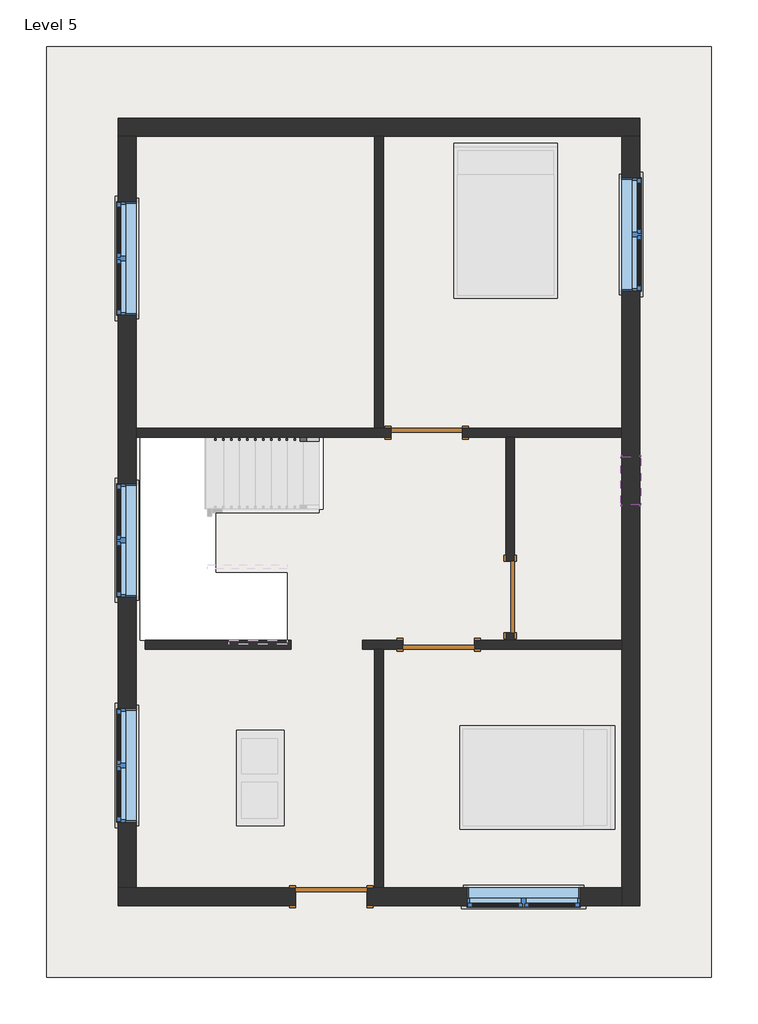
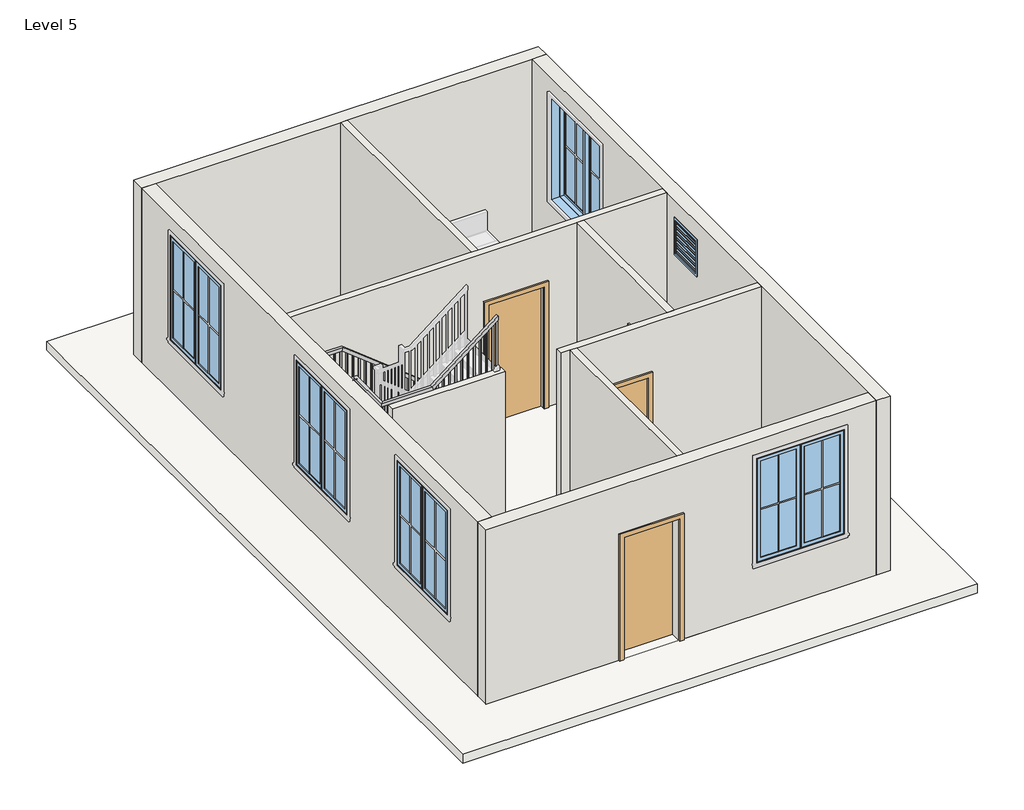
# One storey, part 1 of 2: 10 walls, 6 windows, 4 doors, 1 railing, 1 roof, 1 slab.
"""IFC4 building model written with IfcOpenShell, lengths in millimetres."""

from ifc_helpers import new_model, si_unit, frame, origin, place, context, project, spatial, polyline, outline, extrude, faceted_brep, transform, mapped, element, save
from components import door_e5f9f3c4, door_0ca8825f, window_9ac97e1a, window_f2d8fef0

model = new_model("IFC4")

# Units and contexts
model_context = context("Model", 3, world=origin())
ifc_project = project(units=[si_unit("LENGTHUNIT", "METRE", prefix="MILLI")], contexts=[model_context])

# Site, building, storey
site = spatial("IfcSite", under=ifc_project)
building = spatial("IfcBuilding", under=site)
storey = spatial("IfcBuildingStorey", under=building, Name="Level 5", Elevation=9601.2)

# Doors
placement = place(None, origin())
door_shape = door_e5f9f3c4(model_context)
element("IfcDoor", 1, ObjectType="Single-Flush : 36\" x 84\"", at=placement, inside=storey, context=model_context, shape_type="MappedRepresentation", body=[
    mapped(door_shape, transform((-2225.1840247, 979.1819954, 9601.2), x_axis=(1.0, 0.0, 0.0), y_axis=(0.0, 1.0, 0.0), z_axis=(0.0, 0.0, 1.0))),
])
element("IfcDoor", 2, ObjectType="Single-Flush : 36\" x 84\"", at=placement, inside=storey, context=model_context, shape_type="MappedRepresentation", body=[
    mapped(door_shape, transform((-1158.3840247, -1116.3180046, 9601.2), x_axis=(0.0, -1.0, 0.0), y_axis=(1.0, 0.0, 0.0), z_axis=(0.0, 0.0, 1.0))),
])
element("IfcDoor", 3, ObjectType="Single-Flush : 36\" x 84\"", at=placement, inside=storey, context=model_context, shape_type="MappedRepresentation", body=[
    mapped(door_shape, transform((-2072.7840247, -1725.9180046, 9601.2), x_axis=(-1.0, 0.0, 0.0), y_axis=(0.0, -1.0, 0.0), z_axis=(0.0, 0.0, 1.0))),
])
door_2_shape = door_0ca8825f(model_context)
element("IfcDoor", 4, ObjectType="Single-Flush : 36\" x 84\"", at=placement, inside=storey, context=model_context, shape_type="MappedRepresentation", body=[
    mapped(door_2_shape, transform((-3444.3840247, -4945.3680046, 9601.2), x_axis=(1.0, 0.0, 0.0), y_axis=(0.0, 1.0, 0.0), z_axis=(0.0, 0.0, 1.0))),
])

# Railing
element("IfcRailing", 5, ObjectType="Handrail - Rectangular", at=placement, inside=storey, context=model_context, shape_type="SolidModel", body=[
    faceted_brep([(-3603.1340247, 871.2319954, 10676.0210526), (-3603.1340247, 871.2319954, 10611.2980109), (-3603.1340247, 922.0319954, 10611.2980109), (-3603.1340247, 922.0319954, 10676.0210526), (-5097.5006913, 871.2319954, 11855.7842105), (-5115.1365442, 871.2319954, 11804.9842105), (-5115.1365442, 922.0319954, 11804.9842105), (-5097.5006913, 922.0319954, 11855.7842105), (-5889.1340247, 871.2319954, 11855.7842105), (-5889.1340247, 871.2319954, 11804.9842105), (-5939.9340247, 922.0319954, 11804.9842105), (-5939.9340247, 922.0319954, 11855.7842105), (-5889.1340247, 130.6632454, 11855.7842105), (-5889.1340247, 112.1228815, 11804.9842105), (-5939.9340247, 112.1228815, 11804.9842105), (-5939.9340247, 130.6632454, 11855.7842105), (-5889.1340247, -877.3992546, 12704.6789474), (-5889.1340247, -895.9396185, 12653.8789474), (-5939.9340247, -895.9396185, 12653.8789474), (-5939.9340247, -877.3992546, 12704.6789474), (-5889.1340247, -1617.9680046, 12704.6789474), (-5889.1340247, -1617.9680046, 12653.8789474), (-5939.9340247, -1668.7680046, 12653.8789474), (-5939.9340247, -1668.7680046, 12704.6789474), (-5097.5006913, -1617.9680046, 12704.6789474), (-5079.8648385, -1617.9680046, 12653.8789474), (-5079.8648385, -1668.7680046, 12653.8789474), (-5097.5006913, -1668.7680046, 12704.6789474), (-4009.5340247, -1617.9680046, 13563.6), (-4009.5340247, -1668.7680046, 13563.6), (-4009.5340247, -1668.7680046, 13498.8769583), (-4009.5340247, -1617.9680046, 13498.8769583)], [[[0, 1, 2, 3]], [[1, 0, 4, 5]], [[2, 1, 5, 6]], [[3, 2, 6, 7]], [[0, 3, 7, 4]], [[5, 4, 8, 9]], [[6, 5, 9, 10]], [[7, 6, 10, 11]], [[4, 7, 11, 8]], [[9, 8, 12, 13]], [[10, 9, 13, 14]], [[11, 10, 14, 15]], [[8, 11, 15, 12]], [[13, 12, 16, 17]], [[14, 13, 17, 18]], [[15, 14, 18, 19]], [[12, 15, 19, 16]], [[17, 16, 20, 21]], [[18, 17, 21, 22]], [[19, 18, 22, 23]], [[16, 19, 23, 20]], [[21, 20, 24, 25]], [[22, 21, 25, 26]], [[23, 22, 26, 27]], [[20, 23, 27, 24]], [[28, 29, 30, 31]], [[25, 24, 28, 31]], [[26, 25, 31, 30]], [[27, 26, 30, 29]], [[24, 27, 29, 28]]]),
    extrude(outline(polyline([(13446.2388004, -4076.2090247), (13431.1993267, -4095.2590247), (12488.7789474, -4095.2590247), (12488.7789474, -4076.2090247), (13446.2388004, -4076.2090247)])), frame((0.0, -1652.8930046, 0.0), z_axis=(0.0, 1.0, 0.0), x_axis=(0.0, 0.0, 1.0)), (0.0, 0.0, 1.0), 19.05),
    extrude(outline(polyline([(13366.028274, -4177.8090247), (13350.9888004, -4196.8590247), (12488.7789474, -4196.8590247), (12488.7789474, -4177.8090247), (13366.028274, -4177.8090247)])), frame((0.0, -1652.8930046, 0.0), z_axis=(0.0, 1.0, 0.0), x_axis=(0.0, 0.0, 1.0)), (0.0, 0.0, 1.0), 19.05),
    extrude(outline(polyline([(13285.8177477, -4279.4090247), (13270.778274, -4298.4590247), (12328.3578947, -4298.4590247), (12328.3578947, -4279.4090247), (13285.8177477, -4279.4090247)])), frame((0.0, -1652.8930046, 0.0), z_axis=(0.0, 1.0, 0.0), x_axis=(0.0, 0.0, 1.0)), (0.0, 0.0, 1.0), 19.05),
    extrude(outline(polyline([(13205.6072214, -4381.0090247), (13190.5677477, -4400.0590247), (12328.3578947, -4400.0590247), (12328.3578947, -4381.0090247), (13205.6072214, -4381.0090247)])), frame((0.0, -1652.8930046, 0.0), z_axis=(0.0, 1.0, 0.0), x_axis=(0.0, 0.0, 1.0)), (0.0, 0.0, 1.0), 19.05),
    extrude(outline(polyline([(13125.3966951, -4482.6090247), (13110.3572214, -4501.6590247), (12167.9368421, -4501.6590247), (12167.9368421, -4482.6090247), (13125.3966951, -4482.6090247)])), frame((0.0, -1652.8930046, 0.0), z_axis=(0.0, 1.0, 0.0), x_axis=(0.0, 0.0, 1.0)), (0.0, 0.0, 1.0), 19.05),
    extrude(outline(polyline([(13045.1861688, -4584.2090247), (13030.1466951, -4603.2590247), (12167.9368421, -4603.2590247), (12167.9368421, -4584.2090247), (13045.1861688, -4584.2090247)])), frame((0.0, -1652.8930046, 0.0), z_axis=(0.0, 1.0, 0.0), x_axis=(0.0, 0.0, 1.0)), (0.0, 0.0, 1.0), 19.05),
    extrude(outline(polyline([(12964.9756425, -4685.8090247), (12949.9361688, -4704.8590247), (12007.5157895, -4704.8590247), (12007.5157895, -4685.8090247), (12964.9756425, -4685.8090247)])), frame((0.0, -1652.8930046, 0.0), z_axis=(0.0, 1.0, 0.0), x_axis=(0.0, 0.0, 1.0)), (0.0, 0.0, 1.0), 19.05),
    extrude(outline(polyline([(12884.7651161, -4787.4090247), (12869.7256425, -4806.4590247), (12007.5157895, -4806.4590247), (12007.5157895, -4787.4090247), (12884.7651161, -4787.4090247)])), frame((0.0, -1652.8930046, 0.0), z_axis=(0.0, 1.0, 0.0), x_axis=(0.0, 0.0, 1.0)), (0.0, 0.0, 1.0), 19.05),
    extrude(outline(polyline([(12804.5545898, -4889.0090247), (12789.5151161, -4908.0590247), (11847.0947368, -4908.0590247), (11847.0947368, -4889.0090247), (12804.5545898, -4889.0090247)])), frame((0.0, -1652.8930046, 0.0), z_axis=(0.0, 1.0, 0.0), x_axis=(0.0, 0.0, 1.0)), (0.0, 0.0, 1.0), 19.05),
    extrude(outline(polyline([(12724.3440635, -4990.6090247), (12709.3045898, -5009.6590247), (11847.0947368, -5009.6590247), (11847.0947368, -4990.6090247), (12724.3440635, -4990.6090247)])), frame((0.0, -1652.8930046, 0.0), z_axis=(0.0, 1.0, 0.0), x_axis=(0.0, 0.0, 1.0)), (0.0, 0.0, 1.0), 19.05),
    extrude(outline(polyline([(-5111.2590247, -1652.8930046), (-5111.2590247, -1633.8430046), (-5092.2090247, -1633.8430046), (-5092.2090247, -1652.8930046), (-5111.2590247, -1652.8930046)])), frame((0.0, 0.0, 11686.6736842), z_axis=(0.0, 0.0, 1.0), x_axis=(1.0, 0.0, 0.0)), (0.0, 0.0, 1.0), 967.2052632),
    extrude(outline(polyline([(-5212.8590247, -1652.8930046), (-5212.8590247, -1633.8430046), (-5193.8090247, -1633.8430046), (-5193.8090247, -1652.8930046), (-5212.8590247, -1652.8930046)])), frame((0.0, 0.0, 11686.6736842), z_axis=(0.0, 0.0, 1.0), x_axis=(1.0, 0.0, 0.0)), (0.0, 0.0, 1.0), 967.2052632),
    extrude(outline(polyline([(-5314.4590247, -1652.8930046), (-5314.4590247, -1633.8430046), (-5295.4090247, -1633.8430046), (-5295.4090247, -1652.8930046), (-5314.4590247, -1652.8930046)])), frame((0.0, 0.0, 11686.6736842), z_axis=(0.0, 0.0, 1.0), x_axis=(1.0, 0.0, 0.0)), (0.0, 0.0, 1.0), 967.2052632),
    extrude(outline(polyline([(-5416.0590247, -1652.8930046), (-5416.0590247, -1633.8430046), (-5397.0090247, -1633.8430046), (-5397.0090247, -1652.8930046), (-5416.0590247, -1652.8930046)])), frame((0.0, 0.0, 11686.6736842), z_axis=(0.0, 0.0, 1.0), x_axis=(1.0, 0.0, 0.0)), (0.0, 0.0, 1.0), 967.2052632),
    extrude(outline(polyline([(-5517.6590247, -1652.8930046), (-5517.6590247, -1633.8430046), (-5498.6090247, -1633.8430046), (-5498.6090247, -1652.8930046), (-5517.6590247, -1652.8930046)])), frame((0.0, 0.0, 11686.6736842), z_axis=(0.0, 0.0, 1.0), x_axis=(1.0, 0.0, 0.0)), (0.0, 0.0, 1.0), 967.2052632),
    extrude(outline(polyline([(-5619.2590247, -1652.8930046), (-5619.2590247, -1633.8430046), (-5600.2090247, -1633.8430046), (-5600.2090247, -1652.8930046), (-5619.2590247, -1652.8930046)])), frame((0.0, 0.0, 11686.6736842), z_axis=(0.0, 0.0, 1.0), x_axis=(1.0, 0.0, 0.0)), (0.0, 0.0, 1.0), 967.2052632),
    extrude(outline(polyline([(-5720.8590247, -1652.8930046), (-5720.8590247, -1633.8430046), (-5701.8090247, -1633.8430046), (-5701.8090247, -1652.8930046), (-5720.8590247, -1652.8930046)])), frame((0.0, 0.0, 11686.6736842), z_axis=(0.0, 0.0, 1.0), x_axis=(1.0, 0.0, 0.0)), (0.0, 0.0, 1.0), 967.2052632),
    extrude(outline(polyline([(-5822.4590247, -1652.8930046), (-5822.4590247, -1633.8430046), (-5803.4090247, -1633.8430046), (-5803.4090247, -1652.8930046), (-5822.4590247, -1652.8930046)])), frame((0.0, 0.0, 11686.6736842), z_axis=(0.0, 0.0, 1.0), x_axis=(1.0, 0.0, 0.0)), (0.0, 0.0, 1.0), 967.2052632),
    extrude(outline(polyline([(-5924.0590247, -1532.2430046), (-5905.0090247, -1532.2430046), (-5905.0090247, -1551.2930046), (-5924.0590247, -1551.2930046), (-5924.0590247, -1532.2430046)])), frame((0.0, 0.0, 11686.6736842), z_axis=(0.0, 0.0, 1.0), x_axis=(1.0, 0.0, 0.0)), (0.0, 0.0, 1.0), 967.2052632),
    extrude(outline(polyline([(-5924.0590247, -1430.6430046), (-5905.0090247, -1430.6430046), (-5905.0090247, -1449.6930046), (-5924.0590247, -1449.6930046), (-5924.0590247, -1430.6430046)])), frame((0.0, 0.0, 11686.6736842), z_axis=(0.0, 0.0, 1.0), x_axis=(1.0, 0.0, 0.0)), (0.0, 0.0, 1.0), 967.2052632),
    extrude(outline(polyline([(-5924.0590247, -1329.0430046), (-5905.0090247, -1329.0430046), (-5905.0090247, -1348.0930046), (-5924.0590247, -1348.0930046), (-5924.0590247, -1329.0430046)])), frame((0.0, 0.0, 11686.6736842), z_axis=(0.0, 0.0, 1.0), x_axis=(1.0, 0.0, 0.0)), (0.0, 0.0, 1.0), 967.2052632),
    extrude(outline(polyline([(-5924.0590247, -1227.4430046), (-5905.0090247, -1227.4430046), (-5905.0090247, -1246.4930046), (-5924.0590247, -1246.4930046), (-5924.0590247, -1227.4430046)])), frame((0.0, 0.0, 11686.6736842), z_axis=(0.0, 0.0, 1.0), x_axis=(1.0, 0.0, 0.0)), (0.0, 0.0, 1.0), 967.2052632),
    extrude(outline(polyline([(-5924.0590247, -1125.8430046), (-5905.0090247, -1125.8430046), (-5905.0090247, -1144.8930046), (-5924.0590247, -1144.8930046), (-5924.0590247, -1125.8430046)])), frame((0.0, 0.0, 11686.6736842), z_axis=(0.0, 0.0, 1.0), x_axis=(1.0, 0.0, 0.0)), (0.0, 0.0, 1.0), 967.2052632),
    extrude(outline(polyline([(-5924.0590247, -1024.2430046), (-5905.0090247, -1024.2430046), (-5905.0090247, -1043.2930046), (-5924.0590247, -1043.2930046), (-5924.0590247, -1024.2430046)])), frame((0.0, 0.0, 11686.6736842), z_axis=(0.0, 0.0, 1.0), x_axis=(1.0, 0.0, 0.0)), (0.0, 0.0, 1.0), 967.2052632),
    extrude(outline(polyline([(-5924.0590247, -922.6430046), (-5905.0090247, -922.6430046), (-5905.0090247, -941.6930046), (-5924.0590247, -941.6930046), (-5924.0590247, -922.6430046)])), frame((0.0, 0.0, 11686.6736842), z_axis=(0.0, 0.0, 1.0), x_axis=(1.0, 0.0, 0.0)), (0.0, 0.0, 1.0), 967.2052632),
    extrude(outline(polyline([(-840.0930046, 12606.8502199), (-821.0430046, 12590.8081146), (-821.0430046, 11686.6736842), (-840.0930046, 11686.6736842), (-840.0930046, 12606.8502199)])), frame((-5924.0590247, 0.0, 0.0), z_axis=(1.0, 0.0, 0.0), x_axis=(0.0, 1.0, 0.0)), (0.0, 0.0, 1.0), 19.05),
    extrude(outline(polyline([(-738.4930046, 12521.2923251), (-719.4430046, 12505.2502199), (-719.4430046, 11526.2526316), (-738.4930046, 11526.2526316), (-738.4930046, 12521.2923251)])), frame((-5924.0590247, 0.0, 0.0), z_axis=(1.0, 0.0, 0.0), x_axis=(0.0, 1.0, 0.0)), (0.0, 0.0, 1.0), 19.05),
    extrude(outline(polyline([(-636.8930046, 12435.7344304), (-617.8430046, 12419.6923251), (-617.8430046, 11526.2526316), (-636.8930046, 11526.2526316), (-636.8930046, 12435.7344304)])), frame((-5924.0590247, 0.0, 0.0), z_axis=(1.0, 0.0, 0.0), x_axis=(0.0, 1.0, 0.0)), (0.0, 0.0, 1.0), 19.05),
    extrude(outline(polyline([(-535.2930046, 12350.1765357), (-516.2430046, 12334.1344304), (-516.2430046, 11365.8315789), (-535.2930046, 11365.8315789), (-535.2930046, 12350.1765357)])), frame((-5924.0590247, 0.0, 0.0), z_axis=(1.0, 0.0, 0.0), x_axis=(0.0, 1.0, 0.0)), (0.0, 0.0, 1.0), 19.05),
    extrude(outline(polyline([(-433.6930046, 12264.6186409), (-414.6430046, 12248.5765357), (-414.6430046, 11365.8315789), (-433.6930046, 11365.8315789), (-433.6930046, 12264.6186409)])), frame((-5924.0590247, 0.0, 0.0), z_axis=(1.0, 0.0, 0.0), x_axis=(0.0, 1.0, 0.0)), (0.0, 0.0, 1.0), 19.05),
    extrude(outline(polyline([(-332.0930046, 12179.0607462), (-313.0430046, 12163.0186409), (-313.0430046, 11205.4105263), (-332.0930046, 11205.4105263), (-332.0930046, 12179.0607462)])), frame((-5924.0590247, 0.0, 0.0), z_axis=(1.0, 0.0, 0.0), x_axis=(0.0, 1.0, 0.0)), (0.0, 0.0, 1.0), 19.05),
    extrude(outline(polyline([(-230.4930046, 12093.5028514), (-211.4430046, 12077.4607462), (-211.4430046, 11205.4105263), (-230.4930046, 11205.4105263), (-230.4930046, 12093.5028514)])), frame((-5924.0590247, 0.0, 0.0), z_axis=(1.0, 0.0, 0.0), x_axis=(0.0, 1.0, 0.0)), (0.0, 0.0, 1.0), 19.05),
    extrude(outline(polyline([(-128.8930046, 12007.9449567), (-109.8430046, 11991.9028514), (-109.8430046, 11044.9894737), (-128.8930046, 11044.9894737), (-128.8930046, 12007.9449567)])), frame((-5924.0590247, 0.0, 0.0), z_axis=(1.0, 0.0, 0.0), x_axis=(0.0, 1.0, 0.0)), (0.0, 0.0, 1.0), 19.05),
    extrude(outline(polyline([(-27.2930046, 11922.387062), (-8.2430046, 11906.3449567), (-8.2430046, 11044.9894737), (-27.2930046, 11044.9894737), (-27.2930046, 11922.387062)])), frame((-5924.0590247, 0.0, 0.0), z_axis=(1.0, 0.0, 0.0), x_axis=(0.0, 1.0, 0.0)), (0.0, 0.0, 1.0), 19.05),
    extrude(outline(polyline([(74.3069954, 11836.8291672), (93.3569954, 11820.787062), (93.3569954, 10884.5684211), (74.3069954, 10884.5684211), (74.3069954, 11836.8291672)])), frame((-5924.0590247, 0.0, 0.0), z_axis=(1.0, 0.0, 0.0), x_axis=(0.0, 1.0, 0.0)), (0.0, 0.0, 1.0), 19.05),
    extrude(outline(polyline([(-5924.0590247, 194.9569954), (-5905.0090247, 194.9569954), (-5905.0090247, 175.9069954), (-5924.0590247, 175.9069954), (-5924.0590247, 194.9569954)])), frame((0.0, 0.0, 10884.5684211), z_axis=(0.0, 0.0, 1.0), x_axis=(1.0, 0.0, 0.0)), (0.0, 0.0, 1.0), 920.4157895),
    extrude(outline(polyline([(-5924.0590247, 296.5569954), (-5905.0090247, 296.5569954), (-5905.0090247, 277.5069954), (-5924.0590247, 277.5069954), (-5924.0590247, 296.5569954)])), frame((0.0, 0.0, 10884.5684211), z_axis=(0.0, 0.0, 1.0), x_axis=(1.0, 0.0, 0.0)), (0.0, 0.0, 1.0), 920.4157895),
    extrude(outline(polyline([(-5924.0590247, 398.1569954), (-5905.0090247, 398.1569954), (-5905.0090247, 379.1069954), (-5924.0590247, 379.1069954), (-5924.0590247, 398.1569954)])), frame((0.0, 0.0, 10884.5684211), z_axis=(0.0, 0.0, 1.0), x_axis=(1.0, 0.0, 0.0)), (0.0, 0.0, 1.0), 920.4157895),
    extrude(outline(polyline([(-5924.0590247, 499.7569954), (-5905.0090247, 499.7569954), (-5905.0090247, 480.7069954), (-5924.0590247, 480.7069954), (-5924.0590247, 499.7569954)])), frame((0.0, 0.0, 10884.5684211), z_axis=(0.0, 0.0, 1.0), x_axis=(1.0, 0.0, 0.0)), (0.0, 0.0, 1.0), 920.4157895),
    extrude(outline(polyline([(-5924.0590247, 601.3569954), (-5905.0090247, 601.3569954), (-5905.0090247, 582.3069954), (-5924.0590247, 582.3069954), (-5924.0590247, 601.3569954)])), frame((0.0, 0.0, 10884.5684211), z_axis=(0.0, 0.0, 1.0), x_axis=(1.0, 0.0, 0.0)), (0.0, 0.0, 1.0), 920.4157895),
    extrude(outline(polyline([(-5924.0590247, 702.9569954), (-5905.0090247, 702.9569954), (-5905.0090247, 683.9069954), (-5924.0590247, 683.9069954), (-5924.0590247, 702.9569954)])), frame((0.0, 0.0, 10884.5684211), z_axis=(0.0, 0.0, 1.0), x_axis=(1.0, 0.0, 0.0)), (0.0, 0.0, 1.0), 920.4157895),
    extrude(outline(polyline([(-5924.0590247, 804.5569954), (-5905.0090247, 804.5569954), (-5905.0090247, 785.5069954), (-5924.0590247, 785.5069954), (-5924.0590247, 804.5569954)])), frame((0.0, 0.0, 10884.5684211), z_axis=(0.0, 0.0, 1.0), x_axis=(1.0, 0.0, 0.0)), (0.0, 0.0, 1.0), 920.4157895),
    extrude(outline(polyline([(-5828.8090247, 906.1569954), (-5828.8090247, 887.1069954), (-5847.8590247, 887.1069954), (-5847.8590247, 906.1569954), (-5828.8090247, 906.1569954)])), frame((0.0, 0.0, 10884.5684211), z_axis=(0.0, 0.0, 1.0), x_axis=(1.0, 0.0, 0.0)), (0.0, 0.0, 1.0), 920.4157895),
    extrude(outline(polyline([(-5727.2090247, 906.1569954), (-5727.2090247, 887.1069954), (-5746.2590247, 887.1069954), (-5746.2590247, 906.1569954), (-5727.2090247, 906.1569954)])), frame((0.0, 0.0, 10884.5684211), z_axis=(0.0, 0.0, 1.0), x_axis=(1.0, 0.0, 0.0)), (0.0, 0.0, 1.0), 920.4157895),
    extrude(outline(polyline([(-5625.6090247, 906.1569954), (-5625.6090247, 887.1069954), (-5644.6590247, 887.1069954), (-5644.6590247, 906.1569954), (-5625.6090247, 906.1569954)])), frame((0.0, 0.0, 10884.5684211), z_axis=(0.0, 0.0, 1.0), x_axis=(1.0, 0.0, 0.0)), (0.0, 0.0, 1.0), 920.4157895),
    extrude(outline(polyline([(-5524.0090247, 906.1569954), (-5524.0090247, 887.1069954), (-5543.0590247, 887.1069954), (-5543.0590247, 906.1569954), (-5524.0090247, 906.1569954)])), frame((0.0, 0.0, 10884.5684211), z_axis=(0.0, 0.0, 1.0), x_axis=(1.0, 0.0, 0.0)), (0.0, 0.0, 1.0), 920.4157895),
    extrude(outline(polyline([(-5422.4090247, 906.1569954), (-5422.4090247, 887.1069954), (-5441.4590247, 887.1069954), (-5441.4590247, 906.1569954), (-5422.4090247, 906.1569954)])), frame((0.0, 0.0, 10884.5684211), z_axis=(0.0, 0.0, 1.0), x_axis=(1.0, 0.0, 0.0)), (0.0, 0.0, 1.0), 920.4157895),
    extrude(outline(polyline([(-5320.8090247, 906.1569954), (-5320.8090247, 887.1069954), (-5339.8590247, 887.1069954), (-5339.8590247, 906.1569954), (-5320.8090247, 906.1569954)])), frame((0.0, 0.0, 10884.5684211), z_axis=(0.0, 0.0, 1.0), x_axis=(1.0, 0.0, 0.0)), (0.0, 0.0, 1.0), 920.4157895),
    extrude(outline(polyline([(-5219.2090247, 906.1569954), (-5219.2090247, 887.1069954), (-5238.2590247, 887.1069954), (-5238.2590247, 906.1569954), (-5219.2090247, 906.1569954)])), frame((0.0, 0.0, 10884.5684211), z_axis=(0.0, 0.0, 1.0), x_axis=(1.0, 0.0, 0.0)), (0.0, 0.0, 1.0), 920.4157895),
    extrude(outline(polyline([(-5117.6090247, 906.1569954), (-5117.6090247, 887.1069954), (-5136.6590247, 887.1069954), (-5136.6590247, 906.1569954), (-5117.6090247, 906.1569954)])), frame((0.0, 0.0, 10884.5684211), z_axis=(0.0, 0.0, 1.0), x_axis=(1.0, 0.0, 0.0)), (0.0, 0.0, 1.0), 920.4157895),
    extrude(outline(polyline([(11726.7256425, -5016.0090247), (11741.7651161, -5035.0590247), (10884.5684211, -5035.0590247), (10884.5684211, -5016.0090247), (11726.7256425, -5016.0090247)])), frame((0.0, 887.1069954, 0.0), z_axis=(0.0, 1.0, 0.0), x_axis=(0.0, 0.0, 1.0)), (0.0, 0.0, 1.0), 19.05),
    extrude(outline(polyline([(11646.5151161, -4914.4090247), (11661.5545898, -4933.4590247), (10724.1473684, -4933.4590247), (10724.1473684, -4914.4090247), (11646.5151161, -4914.4090247)])), frame((0.0, 887.1069954, 0.0), z_axis=(0.0, 1.0, 0.0), x_axis=(0.0, 0.0, 1.0)), (0.0, 0.0, 1.0), 19.05),
    extrude(outline(polyline([(11566.3045898, -4812.8090247), (11581.3440635, -4831.8590247), (10724.1473684, -4831.8590247), (10724.1473684, -4812.8090247), (11566.3045898, -4812.8090247)])), frame((0.0, 887.1069954, 0.0), z_axis=(0.0, 1.0, 0.0), x_axis=(0.0, 0.0, 1.0)), (0.0, 0.0, 1.0), 19.05),
    extrude(outline(polyline([(11486.0940635, -4711.2090247), (11501.1335372, -4730.2590247), (10563.7263158, -4730.2590247), (10563.7263158, -4711.2090247), (11486.0940635, -4711.2090247)])), frame((0.0, 887.1069954, 0.0), z_axis=(0.0, 1.0, 0.0), x_axis=(0.0, 0.0, 1.0)), (0.0, 0.0, 1.0), 19.05),
    extrude(outline(polyline([(11405.8835372, -4609.6090247), (11420.9230109, -4628.6590247), (10563.7263158, -4628.6590247), (10563.7263158, -4609.6090247), (11405.8835372, -4609.6090247)])), frame((0.0, 887.1069954, 0.0), z_axis=(0.0, 1.0, 0.0), x_axis=(0.0, 0.0, 1.0)), (0.0, 0.0, 1.0), 19.05),
    extrude(outline(polyline([(11325.6730109, -4508.0090247), (11340.7124846, -4527.0590247), (10403.3052632, -4527.0590247), (10403.3052632, -4508.0090247), (11325.6730109, -4508.0090247)])), frame((0.0, 887.1069954, 0.0), z_axis=(0.0, 1.0, 0.0), x_axis=(0.0, 0.0, 1.0)), (0.0, 0.0, 1.0), 19.05),
    extrude(outline(polyline([(11245.4624846, -4406.4090247), (11260.5019583, -4425.4590247), (10403.3052632, -4425.4590247), (10403.3052632, -4406.4090247), (11245.4624846, -4406.4090247)])), frame((0.0, 887.1069954, 0.0), z_axis=(0.0, 1.0, 0.0), x_axis=(0.0, 0.0, 1.0)), (0.0, 0.0, 1.0), 19.05),
    extrude(outline(polyline([(11165.2519583, -4304.8090247), (11180.2914319, -4323.8590247), (10242.8842105, -4323.8590247), (10242.8842105, -4304.8090247), (11165.2519583, -4304.8090247)])), frame((0.0, 887.1069954, 0.0), z_axis=(0.0, 1.0, 0.0), x_axis=(0.0, 0.0, 1.0)), (0.0, 0.0, 1.0), 19.05),
    extrude(outline(polyline([(11085.0414319, -4203.2090247), (11100.0809056, -4222.2590247), (10242.8842105, -4222.2590247), (10242.8842105, -4203.2090247), (11085.0414319, -4203.2090247)])), frame((0.0, 887.1069954, 0.0), z_axis=(0.0, 1.0, 0.0), x_axis=(0.0, 0.0, 1.0)), (0.0, 0.0, 1.0), 19.05),
    extrude(outline(polyline([(11004.8309056, -4101.6090247), (11019.8703793, -4120.6590247), (10082.4631579, -4120.6590247), (10082.4631579, -4101.6090247), (11004.8309056, -4101.6090247)])), frame((0.0, 887.1069954, 0.0), z_axis=(0.0, 1.0, 0.0), x_axis=(0.0, 0.0, 1.0)), (0.0, 0.0, 1.0), 19.05),
    extrude(outline(polyline([(10924.6203793, -4000.0090247), (10939.659853, -4019.0590247), (10082.4631579, -4019.0590247), (10082.4631579, -4000.0090247), (10924.6203793, -4000.0090247)])), frame((0.0, 887.1069954, 0.0), z_axis=(0.0, 1.0, 0.0), x_axis=(0.0, 0.0, 1.0)), (0.0, 0.0, 1.0), 19.05),
    extrude(outline(polyline([(10844.409853, -3898.4090247), (10859.4493267, -3917.4590247), (9922.0421053, -3917.4590247), (9922.0421053, -3898.4090247), (10844.409853, -3898.4090247)])), frame((0.0, 887.1069954, 0.0), z_axis=(0.0, 1.0, 0.0), x_axis=(0.0, 0.0, 1.0)), (0.0, 0.0, 1.0), 19.05),
    extrude(outline(polyline([(10764.1993267, -3796.8090247), (10779.2388004, -3815.8590247), (9922.0421053, -3815.8590247), (9922.0421053, -3796.8090247), (10764.1993267, -3796.8090247)])), frame((0.0, 887.1069954, 0.0), z_axis=(0.0, 1.0, 0.0), x_axis=(0.0, 0.0, 1.0)), (0.0, 0.0, 1.0), 19.05),
    extrude(outline(polyline([(10683.9888004, -3695.2090247), (10699.028274, -3714.2590247), (9761.6210526, -3714.2590247), (9761.6210526, -3695.2090247), (10683.9888004, -3695.2090247)])), frame((0.0, 887.1069954, 0.0), z_axis=(0.0, 1.0, 0.0), x_axis=(0.0, 0.0, 1.0)), (0.0, 0.0, 1.0), 19.05),
    extrude(outline(polyline([(-5924.0590247, -1633.8430046), (-5905.0090247, -1633.8430046), (-5905.0090247, -1652.8930046), (-5924.0590247, -1652.8930046), (-5924.0590247, -1633.8430046)])), frame((0.0, 0.0, 11686.6736842), z_axis=(0.0, 0.0, 1.0), x_axis=(1.0, 0.0, 0.0)), (0.0, 0.0, 1.0), 967.2052632),
    extrude(outline(polyline([(-5905.0090247, 906.1569954), (-5905.0090247, 887.1069954), (-5924.0590247, 887.1069954), (-5924.0590247, 906.1569954), (-5905.0090247, 906.1569954)])), frame((0.0, 0.0, 10884.5684211), z_axis=(0.0, 0.0, 1.0), x_axis=(1.0, 0.0, 0.0)), (0.0, 0.0, 1.0), 920.4157895),
    extrude(outline(polyline([(13498.8769583, -4009.5340247), (13483.8374846, -4028.5840247), (12488.7789474, -4028.5840247), (12488.7789474, -4009.5340247), (13498.8769583, -4009.5340247)])), frame((0.0, -1652.8930046, 0.0), z_axis=(0.0, 1.0, 0.0), x_axis=(0.0, 0.0, 1.0)), (0.0, 0.0, 1.0), 19.05),
    extrude(outline(polyline([(10611.2980109, -3603.1340247), (10626.3374846, -3622.1840247), (9761.6210526, -3622.1840247), (9761.6210526, -3603.1340247), (10611.2980109, -3603.1340247)])), frame((0.0, 887.1069954, 0.0), z_axis=(0.0, 1.0, 0.0), x_axis=(0.0, 0.0, 1.0)), (0.0, 0.0, 1.0), 19.05),
])

# Roof
element("IfcRoof", 6, ObjectType="ROOF 6\"", at=placement, inside=storey, context=model_context, shape_type="SweptSolid", body=[
    extrude(outline(polyline([(-7082.9340247, 5913.1319954), (1413.3659753, 5913.1319954), (1413.3659753, -5974.0680046), (-7082.9340247, -5974.0680046), (-7082.9340247, 5913.1319954)]), holes=[polyline([(-5889.1340247, 922.0319954), (-5889.1340247, -1668.7680046), (-4009.5340247, -1668.7680046), (-4009.5340247, -805.1680046), (-4923.9340247, -805.1680046), (-4923.9340247, 7.6319954), (-3552.3340247, 7.6319954), (-3552.3340247, 922.0319954), (-5889.1340247, 922.0319954)])]), frame((0.0, 0.0, 9448.8), z_axis=(0.0, 0.0, 1.0), x_axis=(1.0, 0.0, 0.0)), (0.0, 0.0, 1.0), 152.4),
])

# Slab
element("IfcSlab", 7, ObjectType="FLOOR 6\"", at=placement, inside=storey, context=model_context, shape_type="SweptSolid", body=[
    extrude(outline(polyline([(498.9659753, 4998.7319954), (498.9659753, -5059.6680046), (-6168.5340247, -5059.6680046), (-6168.5340247, 4998.7319954), (498.9659753, 4998.7319954)]), holes=[polyline([(-5889.1340247, 922.0319954), (-5889.1340247, -1668.7680046), (-4009.5340247, -1668.7680046), (-4009.5340247, -805.1680046), (-4923.9340247, -805.1680046), (-4923.9340247, 7.6319954), (-3552.3340247, 7.6319954), (-3552.3340247, 922.0319954), (-5889.1340247, 922.0319954)])]), frame((0.0, 0.0, 9448.8), z_axis=(0.0, 0.0, 1.0), x_axis=(1.0, 0.0, 0.0)), (0.0, 0.0, 1.0), 152.4),
])

# Walls
element("IfcWall", 8, ObjectType="WALL 4.5\"", at=placement, inside=storey, context=model_context, shape_type="SweptSolid", body=[
    extrude(outline(polyline([(-2891.9340247, 1036.3319954), (-2891.9340247, 4770.1319954), (-2777.6340247, 4770.1319954), (-2777.6340247, 1036.3319954), (-2891.9340247, 1036.3319954)])), frame((0.0, 0.0, 9601.2), z_axis=(0.0, 0.0, 1.0), x_axis=(1.0, 0.0, 0.0)), (0.0, 0.0, 1.0), 3048.0),
])
element("IfcWall", 9, ObjectType="WALL 4.5\"", at=placement, inside=storey, context=model_context, shape_type="Brep", body=[
    faceted_brep([(-1767.9840247, 922.0319954, 11734.8), (-1767.9840247, 922.0319954, 9601.2), (-1215.5340247, 922.0319954, 9601.2), (-1101.2340247, 922.0319954, 9601.2), (270.3659753, 922.0319954, 9601.2), (270.3659753, 922.0319954, 12649.2), (-1101.2340247, 922.0319954, 12649.2), (-1215.5340247, 922.0319954, 12649.2), (-3552.3340247, 922.0319954, 12649.2), (-5889.1340247, 922.0319954, 12649.2), (-5939.9340247, 922.0319954, 12649.2), (-5939.9340247, 922.0319954, 9601.2), (-2682.3840247, 922.0319954, 9601.2), (-2682.3840247, 922.0319954, 11734.8), (270.3659753, 1036.3319954, 9601.2), (-1767.9840247, 1036.3319954, 9601.2), (-1767.9840247, 1036.3319954, 11734.8), (-2682.3840247, 1036.3319954, 11734.8), (-2682.3840247, 1036.3319954, 9601.2), (-2777.6340247, 1036.3319954, 9601.2), (-2891.9340247, 1036.3319954, 9601.2), (-5939.9340247, 1036.3319954, 9601.2), (-5939.9340247, 1036.3319954, 12649.2), (-2891.9340247, 1036.3319954, 12649.2), (-2777.6340247, 1036.3319954, 12649.2), (270.3659753, 1036.3319954, 12649.2)], [[[0, 1, 2, 3, 4, 5, 6, 7, 8, 9, 10, 11, 12, 13]], [[14, 15, 16, 17, 18, 19, 20, 21, 22, 23, 24, 25]], [[12, 11, 21, 20, 19, 18]], [[4, 3, 2, 1, 15, 14]], [[5, 4, 14, 25]], [[11, 10, 22, 21]], [[16, 15, 1, 0]], [[17, 16, 0, 13]], [[18, 17, 13, 12]], [[10, 9, 8, 7, 6, 5, 25, 24, 23, 22]]]),
])
element("IfcWall", 10, ObjectType="WALL 4.5\"", at=placement, inside=storey, context=model_context, shape_type="SweptSolid", body=[
    extrude(outline(polyline([(-1573.5180046, 11734.8), (-1573.5180046, 9601.2), (-1668.7680046, 9601.2), (-1668.7680046, 12649.2), (922.0319954, 12649.2), (922.0319954, 9601.2), (-659.1180046, 9601.2), (-659.1180046, 11734.8), (-1573.5180046, 11734.8)])), frame((-1215.5340247, 0.0, 0.0), z_axis=(1.0, 0.0, 0.0), x_axis=(0.0, 1.0, 0.0)), (0.0, 0.0, 1.0), 114.3),
])
element("IfcWall", 11, ObjectType="WALL 4.5\"", at=placement, inside=storey, context=model_context, shape_type="Brep", body=[
    faceted_brep([(-2529.9840247, -1668.7680046, 11734.8), (-2529.9840247, -1668.7680046, 9601.2), (-3044.3340247, -1668.7680046, 9601.2), (-3044.3340247, -1668.7680046, 12649.2), (-1215.5340247, -1668.7680046, 12649.2), (-1101.2340247, -1668.7680046, 12649.2), (270.3659753, -1668.7680046, 12649.2), (270.3659753, -1668.7680046, 9601.2), (-1101.2340247, -1668.7680046, 9601.2), (-1215.5340247, -1668.7680046, 9601.2), (-1615.5840247, -1668.7680046, 9601.2), (-1615.5840247, -1668.7680046, 11734.8), (-3044.3340247, -1783.0680046, 9601.2), (-2891.9340247, -1783.0680046, 9601.2), (-2777.6340247, -1783.0680046, 9601.2), (-2529.9840247, -1783.0680046, 9601.2), (-2529.9840247, -1783.0680046, 11734.8), (-1615.5840247, -1783.0680046, 11734.8), (-1615.5840247, -1783.0680046, 9601.2), (270.3659753, -1783.0680046, 9601.2), (270.3659753, -1783.0680046, 12649.2), (-2777.6340247, -1783.0680046, 12649.2), (-2891.9340247, -1783.0680046, 12649.2), (-3044.3340247, -1783.0680046, 12649.2)], [[[0, 1, 2, 3, 4, 5, 6, 7, 8, 9, 10, 11]], [[12, 13, 14, 15, 16, 17, 18, 19, 20, 21, 22, 23]], [[2, 1, 15, 14, 13, 12]], [[10, 9, 8, 7, 19, 18]], [[3, 2, 12, 23]], [[7, 6, 20, 19]], [[16, 15, 1, 0]], [[17, 16, 0, 11]], [[18, 17, 11, 10]], [[6, 5, 4, 3, 23, 22, 21, 20]]]),
])
element("IfcWall", 12, ObjectType="WALL 4.5\"", at=placement, inside=storey, context=model_context, shape_type="Brep", body=[
    faceted_brep([(-5825.6340247, -1783.0680046, 9601.2), (-3958.7340247, -1783.0680046, 9601.2), (-3958.7340247, -1783.0680046, 12649.2), (-5825.6340247, -1783.0680046, 12649.2), (-5825.6340247, -1668.7680046, 9601.2), (-5825.6340247, -1668.7680046, 12649.2), (-4009.5340247, -1668.7680046, 12649.2), (-3958.7340247, -1668.7680046, 12649.2), (-3958.7340247, -1668.7680046, 9601.2)], [[[0, 1, 2, 3]], [[4, 5, 6, 7, 8]], [[1, 0, 4, 8]], [[2, 1, 8, 7]], [[0, 3, 5, 4]], [[3, 2, 7, 6, 5]]]),
])
element("IfcWall", 13, ObjectType="WALL 4.5\"", at=placement, inside=storey, context=model_context, shape_type="SweptSolid", body=[
    extrude(outline(polyline([(-2891.9340247, -4831.0680046), (-2891.9340247, -1783.0680046), (-2777.6340247, -1783.0680046), (-2777.6340247, -4831.0680046), (-2891.9340247, -4831.0680046)])), frame((0.0, 0.0, 9601.2), z_axis=(0.0, 0.0, 1.0), x_axis=(1.0, 0.0, 0.0)), (0.0, 0.0, 1.0), 3048.0),
])
element("IfcWall", 14, ObjectType="WALL 9\"", at=placement, inside=storey, context=model_context, shape_type="Brep", body=[
    faceted_brep([(-6168.5340247, 4770.1319954, 9601.2), (-5939.9340247, 4770.1319954, 9601.2), (-2891.9340247, 4770.1319954, 9601.2), (-2777.6340247, 4770.1319954, 9601.2), (270.3659753, 4770.1319954, 9601.2), (498.9659753, 4770.1319954, 9601.2), (498.9659753, 4770.1319954, 12649.2), (270.3659753, 4770.1319954, 12649.2), (-2777.6340247, 4770.1319954, 12649.2), (-2891.9340247, 4770.1319954, 12649.2), (-5939.9340247, 4770.1319954, 12649.2), (-6168.5340247, 4770.1319954, 12649.2), (-6168.5340247, 4998.7319954, 9601.2), (-6168.5340247, 4998.7319954, 12649.2), (498.9659753, 4998.7319954, 12649.2), (498.9659753, 4998.7319954, 9601.2)], [[[0, 1, 2, 3, 4, 5, 6, 7, 8, 9, 10, 11]], [[12, 13, 14, 15]], [[5, 4, 3, 2, 1, 0, 12, 15]], [[6, 5, 15, 14]], [[0, 11, 13, 12]], [[11, 10, 9, 8, 7, 6, 14, 13]]]),
])
element("IfcWall", 15, ObjectType="WALL 9\"", at=placement, inside=storey, context=model_context, shape_type="Brep", body=[
    faceted_brep([(270.3659753, 4770.1319954, 9601.2), (270.3659753, 1036.3319954, 9601.2), (270.3659753, 922.0319954, 9601.2), (270.3659753, -1668.7680046, 9601.2), (270.3659753, -1783.0680046, 9601.2), (270.3659753, -4831.0680046, 9601.2), (270.3659753, -5059.6680046, 9601.2), (270.3659753, -5059.6680046, 12649.2), (270.3659753, -4831.0680046, 12649.2), (270.3659753, -1783.0680046, 12649.2), (270.3659753, -1668.7680046, 12649.2), (270.3659753, 922.0319954, 12649.2), (270.3659753, 1036.3319954, 12649.2), (270.3659753, 4770.1319954, 12649.2), (270.3659753, 2788.9319954, 12344.4), (270.3659753, 2788.9319954, 10515.6), (270.3659753, 4236.7319954, 10515.6), (270.3659753, 4236.7319954, 12344.4), (270.3659753, 64.7819954, 12344.4), (270.3659753, 64.7819954, 11734.8), (270.3659753, 674.3819954, 11734.8), (270.3659753, 674.3819954, 12344.4), (498.9659753, 4770.1319954, 9601.2), (498.9659753, 4770.1319954, 12649.2), (498.9659753, -5059.6680046, 12649.2), (498.9659753, -5059.6680046, 9601.2), (498.9659753, 2788.9319954, 12344.4), (498.9659753, 4236.7319954, 12344.4), (498.9659753, 4236.7319954, 10515.6), (498.9659753, 2788.9319954, 10515.6), (498.9659753, 64.7819954, 12344.4), (498.9659753, 674.3819954, 12344.4), (498.9659753, 674.3819954, 11734.8), (498.9659753, 64.7819954, 11734.8)], [[[0, 1, 2, 3, 4, 5, 6, 7, 8, 9, 10, 11, 12, 13], [14, 15, 16, 17], [18, 19, 20, 21]], [[22, 23, 24, 25], [26, 27, 28, 29], [30, 31, 32, 33]], [[6, 5, 4, 3, 2, 1, 0, 22, 25]], [[0, 13, 23, 22]], [[7, 6, 25, 24]], [[15, 14, 26, 29]], [[16, 15, 29, 28]], [[17, 16, 28, 27]], [[14, 17, 27, 26]], [[19, 18, 30, 33]], [[20, 19, 33, 32]], [[21, 20, 32, 31]], [[18, 21, 31, 30]], [[13, 12, 11, 10, 9, 8, 7, 24, 23]]]),
])
element("IfcWall", 16, ObjectType="WALL 9\"", at=placement, inside=storey, context=model_context, shape_type="Brep", body=[
    faceted_brep([(270.3659753, -4831.0680046, 9601.2), (-2777.6340247, -4831.0680046, 9601.2), (-2891.9340247, -4831.0680046, 9601.2), (-2987.1840247, -4831.0680046, 9601.2), (-2987.1840247, -4831.0680046, 11734.8), (-3901.5840247, -4831.0680046, 11734.8), (-3901.5840247, -4831.0680046, 9601.2), (-5939.9340247, -4831.0680046, 9601.2), (-6168.5340247, -4831.0680046, 9601.2), (-6168.5340247, -4831.0680046, 12649.2), (-5939.9340247, -4831.0680046, 12649.2), (-2891.9340247, -4831.0680046, 12649.2), (-2777.6340247, -4831.0680046, 12649.2), (270.3659753, -4831.0680046, 12649.2), (-1710.8340247, -4831.0680046, 12344.4), (-1710.8340247, -4831.0680046, 10515.6), (-263.0340247, -4831.0680046, 10515.6), (-263.0340247, -4831.0680046, 12344.4), (-2987.1840247, -5059.6680046, 11734.8), (-2987.1840247, -5059.6680046, 9601.2), (270.3659753, -5059.6680046, 9601.2), (270.3659753, -5059.6680046, 12649.2), (-6168.5340247, -5059.6680046, 12649.2), (-6168.5340247, -5059.6680046, 9601.2), (-3901.5840247, -5059.6680046, 9601.2), (-3901.5840247, -5059.6680046, 11734.8), (-1710.8340247, -5059.6680046, 12344.4), (-263.0340247, -5059.6680046, 12344.4), (-263.0340247, -5059.6680046, 10515.6), (-1710.8340247, -5059.6680046, 10515.6)], [[[0, 1, 2, 3, 4, 5, 6, 7, 8, 9, 10, 11, 12, 13], [14, 15, 16, 17]], [[18, 19, 20, 21, 22, 23, 24, 25], [26, 27, 28, 29]], [[24, 23, 8, 7, 6]], [[20, 19, 3, 2, 1, 0]], [[0, 13, 21, 20]], [[9, 8, 23, 22]], [[15, 14, 26, 29]], [[16, 15, 29, 28]], [[17, 16, 28, 27]], [[14, 17, 27, 26]], [[4, 3, 19, 18]], [[5, 4, 18, 25]], [[6, 5, 25, 24]], [[13, 12, 11, 10, 9, 22, 21]]]),
])
element("IfcWall", 17, ObjectType="WALL 9\"", at=placement, inside=storey, context=model_context, shape_type="Brep", body=[
    faceted_brep([(-5939.9340247, -4831.0680046, 9601.2), (-5939.9340247, 922.0319954, 9601.2), (-5939.9340247, 1036.3319954, 9601.2), (-5939.9340247, 4770.1319954, 9601.2), (-5939.9340247, 4770.1319954, 12649.2), (-5939.9340247, 1036.3319954, 12649.2), (-5939.9340247, 922.0319954, 12649.2), (-5939.9340247, -4831.0680046, 12649.2), (-5939.9340247, -2545.0680046, 12344.4), (-5939.9340247, -2545.0680046, 10515.6), (-5939.9340247, -3992.8680046, 10515.6), (-5939.9340247, -3992.8680046, 12344.4), (-5939.9340247, 3931.9319954, 12344.4), (-5939.9340247, 3931.9319954, 10515.6), (-5939.9340247, 2484.1319954, 10515.6), (-5939.9340247, 2484.1319954, 12344.4), (-5939.9340247, 331.4819954, 12344.4), (-5939.9340247, 331.4819954, 10515.6), (-5939.9340247, -1116.3180046, 10515.6), (-5939.9340247, -1116.3180046, 12344.4), (-6168.5340247, -4831.0680046, 9601.2), (-6168.5340247, -4831.0680046, 12649.2), (-6168.5340247, 4770.1319954, 12649.2), (-6168.5340247, 4770.1319954, 9601.2), (-6168.5340247, -2545.0680046, 12344.4), (-6168.5340247, -3992.8680046, 12344.4), (-6168.5340247, -3992.8680046, 10515.6), (-6168.5340247, -2545.0680046, 10515.6), (-6168.5340247, 3931.9319954, 12344.4), (-6168.5340247, 2484.1319954, 12344.4), (-6168.5340247, 2484.1319954, 10515.6), (-6168.5340247, 3931.9319954, 10515.6), (-6168.5340247, 331.4819954, 12344.4), (-6168.5340247, -1116.3180046, 12344.4), (-6168.5340247, -1116.3180046, 10515.6), (-6168.5340247, 331.4819954, 10515.6)], [[[0, 1, 2, 3, 4, 5, 6, 7], [8, 9, 10, 11], [12, 13, 14, 15], [16, 17, 18, 19]], [[20, 21, 22, 23], [24, 25, 26, 27], [28, 29, 30, 31], [32, 33, 34, 35]], [[3, 2, 1, 0, 20, 23]], [[0, 7, 21, 20]], [[4, 3, 23, 22]], [[9, 8, 24, 27]], [[10, 9, 27, 26]], [[11, 10, 26, 25]], [[8, 11, 25, 24]], [[13, 12, 28, 31]], [[14, 13, 31, 30]], [[15, 14, 30, 29]], [[12, 15, 29, 28]], [[17, 16, 32, 35]], [[18, 17, 35, 34]], [[19, 18, 34, 33]], [[16, 19, 33, 32]], [[7, 6, 5, 4, 22, 21]]]),
])

# Windows
window_shape = window_9ac97e1a(model_context)
element("IfcWindow", 18, ObjectType="Window-Casement-Double : 57\" x 72\"", at=placement, inside=storey, context=model_context, shape_type="MappedRepresentation", body=[
    mapped(window_shape, transform((-986.9340247, -4945.3680046, 9601.2), x_axis=(-1.0, 0.0, 0.0), y_axis=(0.0, -1.0, 0.0), z_axis=(0.0, 0.0, 1.0))),
])
element("IfcWindow", 19, ObjectType="Window-Casement-Double : 57\" x 72\"", at=placement, inside=storey, context=model_context, shape_type="MappedRepresentation", body=[
    mapped(window_shape, transform((-6054.2340247, -3268.9680046, 9601.2), x_axis=(0.0, 1.0, 0.0), y_axis=(-1.0, 0.0, 0.0), z_axis=(0.0, 0.0, 1.0))),
])
element("IfcWindow", 20, ObjectType="Window-Casement-Double : 57\" x 72\"", at=placement, inside=storey, context=model_context, shape_type="MappedRepresentation", body=[
    mapped(window_shape, transform((384.6659753, 3512.8319954, 9601.2), x_axis=(0.0, -1.0, 0.0), y_axis=(1.0, 0.0, 0.0), z_axis=(0.0, 0.0, 1.0))),
])
element("IfcWindow", 21, ObjectType="Window-Casement-Double : 57\" x 72\"", at=placement, inside=storey, context=model_context, shape_type="MappedRepresentation", body=[
    mapped(window_shape, transform((-6054.2340247, 3208.0319954, 9601.2), x_axis=(0.0, 1.0, 0.0), y_axis=(-1.0, 0.0, 0.0), z_axis=(0.0, 0.0, 1.0))),
])
element("IfcWindow", 22, ObjectType="Window-Casement-Double : 57\" x 72\"", at=placement, inside=storey, context=model_context, shape_type="MappedRepresentation", body=[
    mapped(window_shape, transform((-6054.2340247, -392.4180046, 9601.2), x_axis=(0.0, 1.0, 0.0), y_axis=(-1.0, 0.0, 0.0), z_axis=(0.0, 0.0, 1.0))),
])
window_2_shape = window_f2d8fef0(model_context)
element("IfcWindow", 23, ObjectType="Window-Louvers : 24\" x 24\"", at=placement, inside=storey, context=model_context, shape_type="MappedRepresentation", body=[
    mapped(window_2_shape, transform((378.3159753, 369.5819954, 10820.4), x_axis=(0.0, 1.0, 0.0), y_axis=(-1.0, 0.0, 0.0), z_axis=(0.0, 0.0, 1.0))),
])

save(model, "model.ifc")

# Revit data of these elements
# Type "Single-Flush : 36\" x 84\""
#   Type Mark = "1"
#   Construction Type Id = "MDOOR"
#   Assembly Code = "C1020"
#   Analytic Construction = "Metal"
#   Thickness = 0' - 2"
#   Heat Transfer Coefficient (U) = 0.651978 BTU/(h·ft²·°F)
#   Height = 7' - 0"
#   Trim Projection Ext = 0' - 1"
#   Trim Projection Int = 0' - 1"
#   Trim Width = 0' - 3"
#   Width = 3' - 0"
#   Define Thermal Properties by = 1
#   Define Thermal Properties by = 1
#   Door Material = Door - Panel
#   Frame Material = Door - Frame
#   Visual Light Transmittance = 0
#   Solar Heat Gain Coefficient = 0
#   Function = (empty or 0)
#   Wall Closure = (empty or 0)
# Type "Handrail - Rectangular"
#   Assembly Code = "C2010400"
#   built-in parameter 1008612 = 0.0416667 (stored number, unit not read)
#   built-in parameter 1008611 = 0.0416667 (stored number, unit not read)
#   built-in parameter 1008609 = 0.333333 (stored number, unit not read)
#   built-in parameter 1008604 = 0.166667 (stored number, unit not read)
#   built-in parameter 1008603 = 0.166667 (stored number, unit not read)
#   Railing Height = 3' - 0"
#   built-in parameter 1008630 = 2
#   built-in parameter 1008610 = 2
#   built-in parameter 1008618 = Baluster - Square : 3/4"
# Type "ROOF 6\""
#   Assembly Code = "B1020"
#   Layers, outside or top first: 0' - 6" no material (function 1)
# Type "FLOOR 6\""
#   Assembly Code = "B1010"
#   Function = 0
#   Layers, outside or top first: 0' - 6" no material (function 1)
# Type "WALL 4.5\""
#   Assembly Code = "B2010"
#   Layers, outside or top first: 0' - 4 1/2" no material (function 1)
# Type "WALL 9\""
#   Assembly Code = "B2010"
#   Layers, outside or top first: 0' - 9" no material (function 1)
# Type "Window-Casement-Double : 57\" x 72\""
#   Type Mark = "17"
#   Fire Rating = "0.5h"
#   Assembly Code = "B2020100"
#   Analytic Construction = "Double glazing - domestic"
#   Frame Extension [instance default] = 0' - 0 1/4"
#   Window Inset [instance default] = 0' - 0"
#   Wall Thickness [instance default] = 0' - 6"
#   Interior Wall Closure [instance default] = 0' - 2 1/4"
#   Half Width = 2' - 4 1/2"
#   Visual Light Transmittance = 0.81
#   Thermal Resistance (R) = 1.8146 (h·ft²·°F)/BTU
#   Solar Heat Gain Coefficient = 0.76
#   Rough Width = 4' - 9 1/2"
#   Rough Height = 6' - 0 1/2"
#   Height = 6' - 0"
#   Heat Transfer Coefficient (U) = 0.5511 BTU/(h·ft²·°F)
#   Exterior Wall Closure [instance default] = 0' - 1 1/4"
#   Extension Jamb [instance default] = 0' - 2 1/4"
#   Default Sill Height = 3' - 0"
#   Width = 4' - 9"
#   Define Thermal Properties by = 0
#   Muntin Visibility = yes
#   Interior Trim Visibility [instance default] = yes
#   Exterior Trim Visibility [instance default] = yes
#   Extension Jamb Visibility [instance default] = yes
#   Interior Trim Material = Wood - Stained
#   Muntin Pattern = Muntin Pattern_2x2 : Muntin Pattern_2x2
#   Interior Trim = Trim-Window-Interior-Flat : Picture Frame
#   Interior Frame Material = Wood - Stained
#   Glass Panel Material = Glass
#   Exterior Trim Material = Clad - White
#   Exterior Trim = Trim-Window-Exterior-Flat : with Sill
#   Exterior Frame Material = Clad - White
#   Wall Closure = (empty or 0)
# Type "Window-Louvers : 24\" x 24\""
#   Type Mark = "18"
#   Construction Type Id = "GSP4R"
#   Assembly Code = "B20"
#   Analytic Construction = "1/8 in Pilkington single glazing"
#   Visual Light Transmittance = 0.9
#   Thermal Resistance (R) = 1.53941 (h·ft²·°F)/BTU
#   Solar Heat Gain Coefficient = 0.78
#   Max Height = 1' - 11.74264"
#   Height = 2' - 0"
#   Heat Transfer Coefficient (U) = 0.6496 BTU/(h·ft²·°F)
#   Blade Width [instance default] = 1' - 10 1/2"
#   Blade Vertical Thickness = 0' - 0.35355"
#   Blade Thickness = 0' - 0 1/4"
#   Blade Spacing = 0' - 1 1/2"
#   Blade Height = 0' - 1.85355"
#   Blade Depth = 0' - 3"
#   Blade Angle = 45.00°
#   Default Sill Height = 3' - 0"
#   Trim Projection_Exterior = 0' - 0 1/2"
#   Trim Projection_Interior = 0' - 0 1/2"
#   Trim Width_Exterior = 0' - 1 1/2"
#   Trim Width_Interior = 0' - 1 1/2"
#   Width = 2' - 0"
#   Max Blade Count = 12
#   Define Thermal Properties by = 1
#   Blade Count = 12
#   Frame Material = Birch
#   Louver Material = Birch
#   Trim Exterior Material = Birch
#   Trim Interior Material = Birch
#   Wall Closure = (empty or 0)
# Elements 1, 2, 3, 4 (IfcDoor, "Single-Flush : 36\" x 84\"")
#   Phase Created = New Construction
#   Materials on its faces: "Door - Frame", "Door - Panel"
# Element 5 (IfcRailing, "Handrail - Rectangular")
#   Phase Created = New Construction
# Element 6 (IfcRoof, "ROOF 6\"")
#   built-in parameter 1001705 = 31.5 (stored number, unit not read)
#   built-in parameter 1001701 = -0.5 (stored number, unit not read)
#   built-in parameter 1001710 = 33615
#   Phase Created = New Construction
#   Materials on its faces: "Default Roof", "Oak Flooring"
# Element 7 (IfcSlab, "FLOOR 6\"")
#   Height Offset From Level = 0' - 0"
#   Phase Created = New Construction
#   Materials on its faces: "Default Floor"
# Elements 8, 9, 10, 11, 12, 13 (IfcWall, "WALL 4.5\"")
#   Top Offset = 0' - 0"
#   Base Offset = 0' - 0"
#   Unconnected Height = 10' - 0"
#   wall height = 10' - 0"
#   Phase Created = New Construction
#   Base Constraint = Level 5
#   Materials on its faces: "Default Wall"
# Elements 14, 15, 16, 17 (IfcWall, "WALL 9\"")
#   Top Offset = 0' - 0"
#   Base Offset = 0' - 0"
#   Unconnected Height = 10' - 0"
#   wall height = 10' - 0"
#   Phase Created = New Construction
#   Base Constraint = Level 5
#   Materials on its faces: "Default Wall", "Parking Stripe"
# Element 18 (IfcWindow, "Window-Casement-Double : 57\" x 72\"")
#   Mark = "19"
#   Window Inset = 0' - 0"
#   Interior Wall Closure = 0' - 2 1/4"
#   Frame Extension = 0' - 0 1/4"
#   Exterior Wall Closure = 0' - 1 1/4"
#   Interior Trim Visibility = yes
#   Exterior Trim Visibility = yes
#   Phase Created = New Construction
#   Materials on its faces: "Wood - Stained", "Glass", "Clad - White"
# Element 19 (IfcWindow, "Window-Casement-Double : 57\" x 72\"")
#   Mark = "20"
#   Window Inset = 0' - 0"
#   Interior Wall Closure = 0' - 2 1/4"
#   Frame Extension = 0' - 0 1/4"
#   Exterior Wall Closure = 0' - 1 1/4"
#   Interior Trim Visibility = yes
#   Exterior Trim Visibility = yes
#   Phase Created = New Construction
#   Materials on its faces: "Wood - Stained", "Glass", "Clad - White"
# Element 20 (IfcWindow, "Window-Casement-Double : 57\" x 72\"")
#   Mark = "21"
#   Window Inset = 0' - 0"
#   Interior Wall Closure = 0' - 2 1/4"
#   Frame Extension = 0' - 0 1/4"
#   Exterior Wall Closure = 0' - 1 1/4"
#   Interior Trim Visibility = yes
#   Exterior Trim Visibility = yes
#   Phase Created = New Construction
#   Materials on its faces: "Wood - Stained", "Glass", "Clad - White"
# Element 21 (IfcWindow, "Window-Casement-Double : 57\" x 72\"")
#   Mark = "22"
#   Window Inset = 0' - 0"
#   Interior Wall Closure = 0' - 2 1/4"
#   Frame Extension = 0' - 0 1/4"
#   Exterior Wall Closure = 0' - 1 1/4"
#   Interior Trim Visibility = yes
#   Exterior Trim Visibility = yes
#   Phase Created = New Construction
#   Materials on its faces: "Wood - Stained", "Glass", "Clad - White"
# Element 22 (IfcWindow, "Window-Casement-Double : 57\" x 72\"")
#   Mark = "23"
#   Window Inset = 0' - 0"
#   Interior Wall Closure = 0' - 2 1/4"
#   Frame Extension = 0' - 0 1/4"
#   Exterior Wall Closure = 0' - 1 1/4"
#   Interior Trim Visibility = yes
#   Exterior Trim Visibility = yes
#   Phase Created = New Construction
#   Materials on its faces: "Wood - Stained", "Glass", "Clad - White"
# Element 23 (IfcWindow, "Window-Louvers : 24\" x 24\"")
#   Mark = "24"
#   Blade Width = 1' - 10 1/2"
#   Phase Created = New Construction
#   Materials on its faces: "Birch"
# Materials
#   "Door - Panel": class "Wood", colour RGB 210 159 95, transparency 0, Cost = 0
#   "Door - Frame": colour RGB 118 70 51, transparency 0, Cost = 0
#   "Wood - Stained": class "Wood", colour RGB 224 178 126, transparency 0, Cost = 0
#   "Glass": class "Glass", colour RGB 0 128 192, transparency 0.75, Description = "Soda Lime Glass", Cost = 0
#   "Clad - White": class "Wood", colour RGB 242 242 238, transparency 0, Cost = 0
#   "Birch": class "Wood", colour RGB 224 178 126, transparency 0, Description = "Betula Alleghaniensis", Cost = 0
#   "Default Roof": colour RGB 88 101 114, transparency 0, Cost = 0
#   "Oak Flooring": class "Wood", colour RGB 216 169 114, transparency 0, Description = "Quercus Rubra", Cost = 0
#   "Default Floor": colour RGB 128 128 128, transparency 0, Cost = 0
#   "Default Wall": colour RGB 128 128 128, transparency 0, Cost = 0
#   "Parking Stripe": class "Paint", colour RGB 250 250 91, transparency 0, Cost = 0
